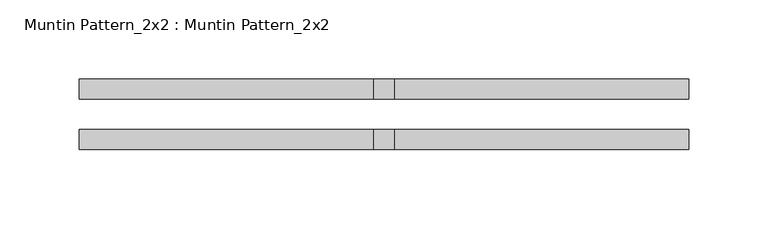
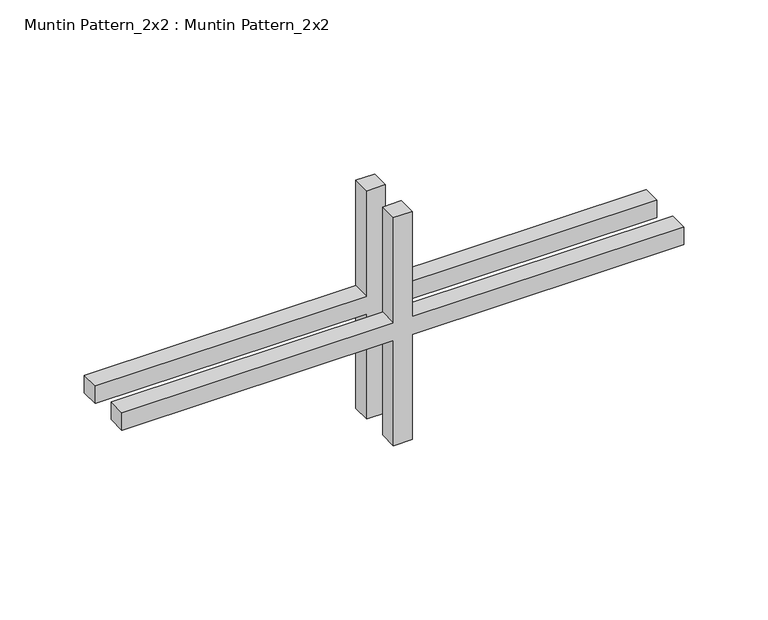
"""IFC4 building model written with IfcOpenShell, lengths in millimetres: proxy geometry, Muntin Pattern_2x2 : Muntin Pattern_2x2."""

from ifc_helpers import new_model, si_unit, frame, origin, place, context, project, spatial, polyline, outline, extrude, source, transform, mapped, element, save


def muntin_pattern_2x2_muntin_pattern_2x2_4879a4f3(model_context):
    return source(origin(), model_context, "Body", "SweptSolid", [
        extrude(outline(polyline([(88.9, -6.35), (88.9, -192.0875), (76.2, -192.0875), (76.2, -6.35), (0.0, -6.35), (0.0, 6.35), (76.2, 6.35), (76.2, 192.0875), (88.9, 192.0875), (88.9, 6.35), (165.1, 6.35), (165.1, -6.35), (88.9, -6.35)])), frame((0.0, -22.225, 0.0), z_axis=(0.0, 1.0, 0.0), x_axis=(0.0, 0.0, 1.0)), (0.0, 0.0, 1.0), 12.7),
        extrude(outline(polyline([(88.9, -6.35), (88.9, -192.0875), (76.2, -192.0875), (76.2, -6.35), (0.0, -6.35), (0.0, 6.35), (76.2, 6.35), (76.2, 192.0875), (88.9, 192.0875), (88.9, 6.35), (165.1, 6.35), (165.1, -6.35), (88.9, -6.35)])), frame((0.0, 9.525, 0.0), z_axis=(0.0, 1.0, 0.0), x_axis=(0.0, 0.0, 1.0)), (0.0, 0.0, 1.0), 12.7),
    ])


if __name__ == "__main__":
    model = new_model("IFC4")
    model_context = context("Model", 3, world=origin())
    ifc_project = project(units=[si_unit("LENGTHUNIT", "METRE", prefix="MILLI")], contexts=[model_context])
    site = spatial("IfcSite", under=ifc_project)
    building = spatial("IfcBuilding", under=site)
    placement = place(None, origin())
    muntin_pattern_2x2_muntin_pattern_2x2_shape = muntin_pattern_2x2_muntin_pattern_2x2_4879a4f3(model_context)
    element("IfcBuildingElementProxy", 1, Name="Muntin Pattern_2x2 : Muntin Pattern_2x2", ObjectType="Muntin Pattern_2x2 : Muntin Pattern_2x2", at=placement, inside=building, context=model_context, shape_type="MappedRepresentation", body=[
        mapped(muntin_pattern_2x2_muntin_pattern_2x2_shape, transform((0.0, 0.0, 0.0), x_axis=(1.0, 0.0, 0.0), y_axis=(0.0, 1.0, 0.0), z_axis=(0.0, 0.0, 1.0))),
    ])
    save(model, "model.ifc")

# Revit data of these elements
# Type "Muntin Pattern_2x2 : Muntin Pattern_2x2"
#   Width [instance default] = 4' - 0"
#   Thickness = 0' - 0 1/2"
#   Height [instance default] = 4' - 0"
#   Distance = 0' - 0 3/4"
#   Interior Material [instance default] = none
#   Exterior Material [instance default] = none
#   Default Elevation = 0
# Element 1 (IfcBuildingElementProxy, "Muntin Pattern_2x2 : Muntin Pattern_2x2")
#   Width = 1' - 3 1/8"
#   Height = 0' - 6 1/2"
#   Interior Material = Wood - Stained
#   Exterior Material = Clad - White
#   Materials on its faces: "Clad - White", "Wood - Stained"
# Materials
#   "Clad - White": class "Wood", colour RGB 242 242 238, transparency 0, Cost = 0
#   "Wood - Stained": class "Wood", colour RGB 224 178 126, transparency 0, Cost = 0
